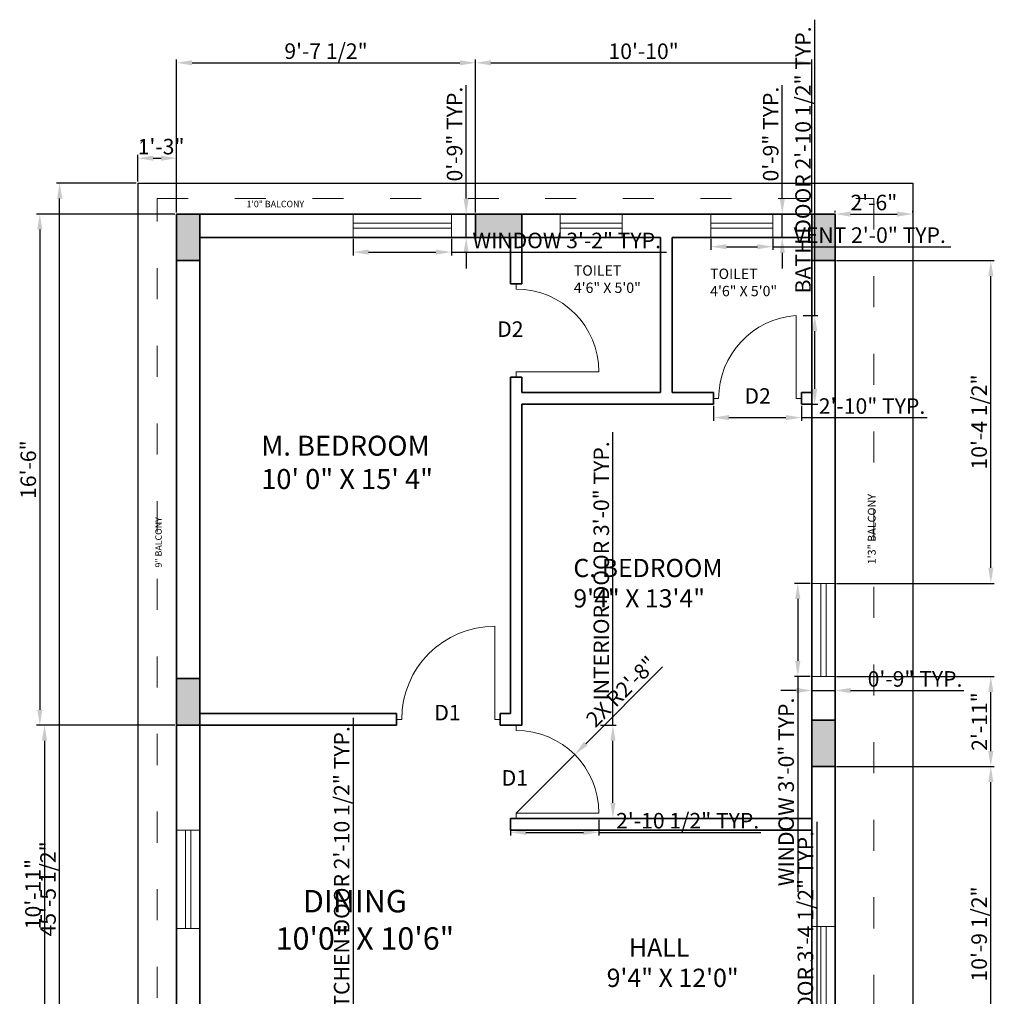
# Model space of a CAD drawing. Units: inches. Extents: x 40559 to 41508, y 131086 to 132358.
# Tile 4 of 5: x 41128 to 41508, y 131353 to 131730. Entities that reach past the tile are written whole.
import ezdxf

# ---------------------------------------------------------------- set-up
doc = ezdxf.new("R2010")
doc.units = ezdxf.units.IN
doc.linetypes.add('ACAD_ISO03W100', pattern=[30, 12, -18])
for name, color, linetype, lineweight in [('A-ANNO-DIMS', 2, 'Continuous', 18), ('A-ANNO-TEXT', 7, 'Continuous', 18), ('A-AREA-IDEN', 7, 'Continuous', 18), ('A-FLOR-FIXT', 4, 'Continuous', 18), ('A-FLOR-OVHD', 240, 'ACAD_ISO03W100', 13), ('A-WALL', 7, 'Continuous', 35), ('C-PROP', 7, 'Continuous', 25), ('Doors', 50, 'Continuous', 18), ('Windows', 70, 'Continuous', 18)]:
    doc.layers.add(name, color=color, linetype=linetype, lineweight=lineweight)
doc.layers.add('A-COLS', color=177, linetype='Continuous', lineweight=35, true_color=0x293189)
doc.styles.get("Standard").update_dxf_attribs({"font": 'arial.ttf'})
doc.dimstyles.new('ISO-25', dxfattribs={"dimtxt": 6, "dimasz": 6, "dimexe": 1.25, "dimexo": 0.625, "dimtad": 1, "dimdec": 0, "dimlunit": 3, "dimtxsty": 'Standard', "dimcen": 2.5, "dimclrd": 1, "dimclre": 1, "dimclrt": 2, "dimadec": 0, "dimazin": 0, "dimtfac": 1, "dimtdec": 0, "dimtmove": 0, "dimatfit": 3, "dimfxl": 1, "dimarcsym": 0})

# ---------------------------------------------------------------- blocks, each defined once
blk = doc.blocks.new('*D1')
at = {"layer": 'A-ANNO-DIMS', "color": 0, "lineweight": -2, "transparency": 16777216}
for p, q in [((41173.52, 131667.98), (41173.52, 131678.2)), ((41179.52, 131676.95), (41182.52, 131676.95)), ((41188.52, 131667.98), (41188.52, 131678.2))]:
    blk.add_line(p, q, dxfattribs=at)
at = {"layer": 'A-ANNO-DIMS', "color": 0, "transparency": 16777216}
for points in [[(41179.52, 131677.95), (41179.52, 131675.95), (41173.52, 131676.95)], [(41182.52, 131677.95), (41182.52, 131675.95), (41188.52, 131676.95)]]:
    blk.add_solid(points, dxfattribs=at)
at = {"layer": 'Defpoints', "color": 0, "transparency": 16777216}
for p in [(41188.52, 131676.95), (41173.52, 131667.35), (41188.52, 131667.35)]:
    blk.add_point(p, dxfattribs=at)
at = {"layer": 'A-ANNO-DIMS', "color": 0, "transparency": 16777216, "insert": (41182.52, 131680.64), "char_height": 6, "attachment_point": 5}
blk.add_mtext('1\'-3"', dxfattribs=at)
blk = doc.blocks.new('*D2')
at = {"layer": 'A-ANNO-DIMS', "color": 0, "lineweight": -2, "transparency": 16777216}
for p, q in [((41187.89, 131655.35), (41134.4, 131655.35)), ((41135.65, 131649.35), (41135.65, 131463.85)), ((41187.89, 131457.85), (41134.4, 131457.85))]:
    blk.add_line(p, q, dxfattribs=at)
at = {"layer": 'A-ANNO-DIMS', "color": 0, "transparency": 16777216}
for points in [[(41134.65, 131649.35), (41136.65, 131649.35), (41135.65, 131655.35)], [(41134.65, 131463.85), (41136.65, 131463.85), (41135.65, 131457.85)]]:
    blk.add_solid(points, dxfattribs=at)
at = {"layer": 'Defpoints', "color": 0, "transparency": 16777216}
for p in [(41188.52, 131655.35), (41135.65, 131457.85), (41188.52, 131457.85)]:
    blk.add_point(p, dxfattribs=at)
at = {"layer": 'A-ANNO-DIMS', "color": 0, "transparency": 16777216, "insert": (41131.96, 131556.6), "char_height": 6, "attachment_point": 5, "rotation": 90}
blk.add_mtext('16\'-6"', dxfattribs=at)
blk = doc.blocks.new('*D3')
at = {"layer": 'A-ANNO-DIMS', "color": 0, "lineweight": -2, "transparency": 16777216}
for p, q in [((41187.89, 131457.85), (41136.22, 131457.85)), ((41137.47, 131451.85), (41137.47, 131333.35)), ((41196.89, 131327.35), (41136.22, 131327.35))]:
    blk.add_line(p, q, dxfattribs=at)
at = {"layer": 'A-ANNO-DIMS', "color": 0, "transparency": 16777216}
for points in [[(41136.47, 131451.85), (41138.47, 131451.85), (41137.47, 131457.85)], [(41136.47, 131333.35), (41138.47, 131333.35), (41137.47, 131327.35)]]:
    blk.add_solid(points, dxfattribs=at)
at = {"layer": 'Defpoints', "color": 0, "transparency": 16777216}
for p in [(41188.52, 131457.85), (41137.47, 131327.35), (41197.52, 131327.35)]:
    blk.add_point(p, dxfattribs=at)
at = {"layer": 'A-ANNO-DIMS', "color": 0, "transparency": 16777216, "insert": (41133.78, 131392.6), "char_height": 6, "attachment_point": 5, "rotation": 90}
blk.add_mtext('10\'-11"', dxfattribs=at)
blk = doc.blocks.new('*D5')
at = {"layer": 'A-ANNO-DIMS', "color": 0, "lineweight": -2, "transparency": 16777216}
for p, q in [((41443.02, 131655.98), (41443.02, 131656.6)), ((41473.02, 131655.98), (41473.02, 131656.6)), ((41449.02, 131655.35), (41467.02, 131655.35))]:
    blk.add_line(p, q, dxfattribs=at)
at = {"layer": 'A-ANNO-DIMS', "color": 0, "transparency": 16777216}
for points in [[(41449.02, 131656.35), (41449.02, 131654.35), (41443.02, 131655.35)], [(41467.02, 131656.35), (41467.02, 131654.35), (41473.02, 131655.35)]]:
    blk.add_solid(points, dxfattribs=at)
at = {"layer": 'Defpoints', "color": 0, "transparency": 16777216}
for p in [(41443.02, 131655.35), (41473.02, 131655.35), (41473.02, 131655.35)]:
    blk.add_point(p, dxfattribs=at)
at = {"layer": 'A-ANNO-DIMS', "color": 0, "transparency": 16777216, "insert": (41458.02, 131659.04), "char_height": 6, "attachment_point": 5}
blk.add_mtext('2\'-6"', dxfattribs=at)
blk = doc.blocks.new('WIN-36IN')
for p, q in [((0, 5.5), (36, 5.5)), ((0, 3.5), (36, 3.5))]:
    blk.add_line(p, q)
blk.add_lwpolyline([(0, 9), (36, 9), (36, 0), (0, 0)], close=True)
blk = doc.blocks.new('WIN-38IN')
for p, q in [((0, 5.5), (38, 5.5)), ((0, 3.5), (38, 3.5))]:
    blk.add_line(p, q)
blk.add_lwpolyline([(0, 9), (38, 9), (38, 0), (0, 0)], close=True)
blk = doc.blocks.new('VENT-24IN')
for p, q in [((0, 5.5), (24, 5.5)), ((0, 3.5), (24, 3.5))]:
    blk.add_line(p, q)
blk.add_lwpolyline([(0, 9), (24, 9), (24, 0), (0, 0)], close=True)
blk = doc.blocks.new('DOOR-INT-36IN')
for p, q in [((2.25, 34), (2.25, 36)), ((4.5, 0), (0, 0)), ((2.25, 0), (2.25, 2)), ((2.25, 2), (34.25, 2))]:
    blk.add_line(p, q)
blk.add_arc((2.25, 2), 32, 0, 90)
blk = doc.blocks.new('DOOR-BATH-34IN')
for p, q in [((32, 2.25), (32, 34.25)), ((34, 4.5), (34, 0)), ((0, 2.25), (2, 2.25)), ((34, 2.25), (32, 2.25))]:
    blk.add_line(p, q)
blk.add_arc((34.07, 2.25), 32.07, 93.6952, 180)
blk = doc.blocks.new('DOOR-INT-40IN')
for p, q in [((38, 2.25), (38, 38.25)), ((40, 4.5), (40, 0)), ((2, 2.25), (0, 2.25)), ((40, 2.25), (38, 2.25))]:
    blk.add_line(p, q)
blk.add_arc((38, 2.25), 36, 90, 180)
blk = doc.blocks.new('COL-9X18IN')
h = blk.add_hatch(color=256)
h.dxf.hatch_style = 1
h.paths.add_polyline_path([(9, 18), (0, 18), (0, 0), (9, 0)])
blk.add_lwpolyline([(0, 18), (9, 18), (9, 0), (0, 0)], close=True)
blk = doc.blocks.new('*D34')
at = {"layer": 'A-ANNO-DIMS', "color": 1, "lineweight": -2, "transparency": 16777216}
for p, q in [((41433.39, 131512.67), (41427.37, 131512.67)), ((41428.62, 131506.67), (41428.62, 131482.67)), ((41433.39, 131476.67), (41427.37, 131476.67)), ((41428.62, 131476.67), (41428.62, 131393.5))]:
    blk.add_line(p, q, dxfattribs=at)
at = {"layer": 'A-ANNO-DIMS', "color": 1, "transparency": 16777216}
for points in [[(41427.62, 131506.67), (41429.62, 131506.67), (41428.62, 131512.67)], [(41427.62, 131482.67), (41429.62, 131482.67), (41428.62, 131476.67)]]:
    blk.add_solid(points, dxfattribs=at)
at = {"layer": 'Defpoints', "color": 0, "transparency": 16777216}
for p in [(41434.02, 131512.67), (41428.62, 131476.67), (41434.02, 131476.67)]:
    blk.add_point(p, dxfattribs=at)
at = {"layer": 'A-ANNO-DIMS', "color": 2, "transparency": 16777216, "insert": (41424.89, 131432.08), "char_height": 6, "attachment_point": 5, "rotation": 90}
blk.add_mtext('WINDOW 3\'-0" TYP.', dxfattribs=at)
blk = doc.blocks.new('*D35')
at = {"layer": 'A-ANNO-DIMS', "color": 1, "lineweight": -2, "transparency": 16777216}
for p, q in [((41434.02, 131476.05), (41434.02, 131470.02)), ((41443.02, 131476.05), (41443.02, 131470.02)), ((41428.02, 131471.27), (41422.02, 131471.27)), ((41434.02, 131471.27), (41443.02, 131471.27)), ((41449.02, 131471.27), (41492.84, 131471.27))]:
    blk.add_line(p, q, dxfattribs=at)
at = {"layer": 'A-ANNO-DIMS', "color": 1, "transparency": 16777216}
for points in [[(41428.02, 131472.27), (41428.02, 131470.27), (41434.02, 131471.27)], [(41449.02, 131472.27), (41449.02, 131470.27), (41443.02, 131471.27)]]:
    blk.add_solid(points, dxfattribs=at)
at = {"layer": 'Defpoints', "color": 0, "transparency": 16777216}
for p in [(41434.02, 131476.67), (41443.02, 131476.67), (41443.02, 131471.27)]:
    blk.add_point(p, dxfattribs=at)
at = {"layer": 'A-ANNO-DIMS', "color": 2, "transparency": 16777216, "insert": (41473.93, 131474.96), "char_height": 6, "attachment_point": 5}
blk.add_mtext('0\'-9" TYP.', dxfattribs=at)
blk = doc.blocks.new('*D36')
at = {"layer": 'A-ANNO-DIMS', "color": 1, "lineweight": -2, "transparency": 16777216}
for p, q in [((41256.73, 131645.73), (41256.73, 131639.4)), ((41294.73, 131645.73), (41294.73, 131639.4)), ((41262.73, 131640.65), (41288.73, 131640.65)), ((41294.73, 131640.65), (41377.9, 131640.65))]:
    blk.add_line(p, q, dxfattribs=at)
at = {"layer": 'A-ANNO-DIMS', "color": 1, "transparency": 16777216}
for points in [[(41262.73, 131641.65), (41262.73, 131639.65), (41256.73, 131640.65)], [(41288.73, 131641.65), (41288.73, 131639.65), (41294.73, 131640.65)]]:
    blk.add_solid(points, dxfattribs=at)
at = {"layer": 'Defpoints', "color": 0, "transparency": 16777216}
for p in [(41256.73, 131646.35), (41294.73, 131646.35), (41294.73, 131640.65)]:
    blk.add_point(p, dxfattribs=at)
at = {"layer": 'A-ANNO-DIMS', "color": 2, "transparency": 16777216, "insert": (41339.31, 131644.38), "char_height": 6, "attachment_point": 5}
blk.add_mtext('WINDOW 3\'-2" TYP.', dxfattribs=at)
blk = doc.blocks.new('*D37')
at = {"layer": 'A-ANNO-DIMS', "color": 1, "lineweight": -2, "transparency": 16777216}
for p, q in [((41300.43, 131661.35), (41300.43, 131705.17)), ((41295.35, 131655.35), (41301.68, 131655.35)), ((41300.43, 131646.35), (41300.43, 131655.35)), ((41295.35, 131646.35), (41301.68, 131646.35)), ((41300.43, 131640.35), (41300.43, 131634.35))]:
    blk.add_line(p, q, dxfattribs=at)
at = {"layer": 'A-ANNO-DIMS', "color": 1, "transparency": 16777216}
for points in [[(41299.43, 131661.35), (41301.43, 131661.35), (41300.43, 131655.35)], [(41299.43, 131640.35), (41301.43, 131640.35), (41300.43, 131646.35)]]:
    blk.add_solid(points, dxfattribs=at)
at = {"layer": 'Defpoints', "color": 0, "transparency": 16777216}
for p in [(41294.73, 131655.35), (41300.43, 131655.35), (41294.73, 131646.35)]:
    blk.add_point(p, dxfattribs=at)
at = {"layer": 'A-ANNO-DIMS', "color": 2, "transparency": 16777216, "insert": (41296.74, 131686.26), "char_height": 6, "attachment_point": 5, "rotation": 90}
blk.add_mtext('0\'-9" TYP.', dxfattribs=at)
blk = doc.blocks.new('*D38')
at = {"layer": 'A-ANNO-DIMS', "color": 1, "lineweight": -2, "transparency": 16777216}
for p, q in [((41395.02, 131645.73), (41395.02, 131641.5)), ((41419.02, 131645.73), (41419.02, 131641.5)), ((41401.02, 131642.75), (41413.02, 131642.75)), ((41419.02, 131642.75), (41487.83, 131642.75))]:
    blk.add_line(p, q, dxfattribs=at)
at = {"layer": 'A-ANNO-DIMS', "color": 1, "transparency": 16777216}
for points in [[(41401.02, 131643.75), (41401.02, 131641.75), (41395.02, 131642.75)], [(41413.02, 131643.75), (41413.02, 131641.75), (41419.02, 131642.75)]]:
    blk.add_solid(points, dxfattribs=at)
at = {"layer": 'Defpoints', "color": 0, "transparency": 16777216}
for p in [(41395.02, 131646.35), (41419.02, 131646.35), (41419.02, 131642.75)]:
    blk.add_point(p, dxfattribs=at)
at = {"layer": 'A-ANNO-DIMS', "color": 2, "transparency": 16777216, "insert": (41456.43, 131646.44), "char_height": 6, "attachment_point": 5}
blk.add_mtext('VENT 2\'-0" TYP.', dxfattribs=at)
blk = doc.blocks.new('*D39')
at = {"layer": 'A-ANNO-DIMS', "color": 1, "lineweight": -2, "transparency": 16777216}
for p, q in [((41422.62, 131661.35), (41422.62, 131705.17)), ((41419.64, 131655.35), (41423.87, 131655.35)), ((41422.62, 131646.35), (41422.62, 131655.35)), ((41419.64, 131646.35), (41423.87, 131646.35)), ((41422.62, 131640.35), (41422.62, 131634.35))]:
    blk.add_line(p, q, dxfattribs=at)
at = {"layer": 'A-ANNO-DIMS', "color": 1, "transparency": 16777216}
for points in [[(41421.62, 131661.35), (41423.62, 131661.35), (41422.62, 131655.35)], [(41421.62, 131640.35), (41423.62, 131640.35), (41422.62, 131646.35)]]:
    blk.add_solid(points, dxfattribs=at)
at = {"layer": 'Defpoints', "color": 0, "transparency": 16777216}
for p in [(41419.02, 131655.35), (41422.62, 131655.35), (41419.02, 131646.35)]:
    blk.add_point(p, dxfattribs=at)
at = {"layer": 'A-ANNO-DIMS', "color": 2, "transparency": 16777216, "insert": (41418.93, 131686.26), "char_height": 6, "attachment_point": 5, "rotation": 90}
blk.add_mtext('0\'-9" TYP.', dxfattribs=at)
blk = doc.blocks.new('*D40')
at = {"layer": 'A-ANNO-DIMS', "color": 1, "lineweight": -2, "transparency": 16777216}
for p, q in [((41357.17, 131457.85), (41357.17, 131571.09)), ((41352.39, 131457.85), (41358.42, 131457.85)), ((41357.17, 131427.85), (41357.17, 131451.85)), ((41352.39, 131421.85), (41358.42, 131421.85))]:
    blk.add_line(p, q, dxfattribs=at)
at = {"layer": 'A-ANNO-DIMS', "color": 1, "transparency": 16777216}
for points in [[(41356.17, 131451.85), (41358.17, 131451.85), (41357.17, 131457.85)], [(41356.17, 131427.85), (41358.17, 131427.85), (41357.17, 131421.85)]]:
    blk.add_solid(points, dxfattribs=at)
at = {"layer": 'Defpoints', "color": 0, "transparency": 16777216}
for p in [(41351.77, 131457.85), (41357.17, 131457.85), (41351.77, 131421.85)]:
    blk.add_point(p, dxfattribs=at)
at = {"layer": 'A-ANNO-DIMS', "color": 2, "transparency": 16777216, "insert": (41353.44, 131517.47), "char_height": 6, "attachment_point": 5, "rotation": 90}
blk.add_mtext('INTERIOR DOOR 3\'-0" TYP.', dxfattribs=at)
blk = doc.blocks.new('*D41')
at = {"layer": 'A-ANNO-DIMS', "color": 1, "lineweight": -2, "transparency": 16777216}
for p, q in [((41317.52, 131421.23), (41317.52, 131415.2)), ((41351.77, 131421.23), (41351.77, 131415.2)), ((41323.52, 131416.45), (41345.77, 131416.45)), ((41351.77, 131416.45), (41414.33, 131416.45))]:
    blk.add_line(p, q, dxfattribs=at)
at = {"layer": 'A-ANNO-DIMS', "color": 1, "transparency": 16777216}
for points in [[(41323.52, 131417.45), (41323.52, 131415.45), (41317.52, 131416.45)], [(41345.77, 131417.45), (41345.77, 131415.45), (41351.77, 131416.45)]]:
    blk.add_solid(points, dxfattribs=at)
at = {"layer": 'Defpoints', "color": 0, "transparency": 16777216}
for p in [(41317.52, 131421.85), (41351.77, 131421.85), (41351.77, 131416.45)]:
    blk.add_point(p, dxfattribs=at)
at = {"layer": 'A-ANNO-DIMS', "color": 2, "transparency": 16777216, "insert": (41386.05, 131420.18), "char_height": 6, "attachment_point": 5}
blk.add_mtext('2\'-10 1/2" TYP.', dxfattribs=at)
blk = doc.blocks.new('*D42')
at = {"layer": 'A-ANNO-DIMS', "color": 1, "lineweight": -2, "transparency": 16777216}
for p, q in [((41256.84, 131331.85), (41256.84, 131460.64)), ((41261.35, 131331.85), (41255.59, 131331.85)), ((41256.84, 131303.6), (41256.84, 131325.85)), ((41261.35, 131297.6), (41255.59, 131297.6))]:
    blk.add_line(p, q, dxfattribs=at)
at = {"layer": 'A-ANNO-DIMS', "color": 1, "transparency": 16777216}
for points in [[(41255.84, 131325.85), (41257.84, 131325.85), (41256.84, 131331.85)], [(41255.84, 131303.6), (41257.84, 131303.6), (41256.84, 131297.6)]]:
    blk.add_solid(points, dxfattribs=at)
at = {"layer": 'Defpoints', "color": 0, "transparency": 16777216}
for p in [(41256.84, 131331.85), (41261.98, 131331.85), (41261.98, 131297.6)]:
    blk.add_point(p, dxfattribs=at)
at = {"layer": 'A-ANNO-DIMS', "color": 2, "transparency": 16777216, "insert": (41253.11, 131399.25), "char_height": 6, "attachment_point": 5, "rotation": 90}
blk.add_mtext('KITCHEN DOOR 2\'-10 1/2" TYP.', dxfattribs=at)
blk = doc.blocks.new('*D44')
at = {"layer": 'A-ANNO-DIMS', "color": 1, "lineweight": -2, "transparency": 16777216}
for p, q in [((41436.09, 131304.85), (41436.09, 131420.55)), ((41430.64, 131304.85), (41437.34, 131304.85)), ((41436.09, 131270.35), (41436.09, 131298.85)), ((41430.64, 131264.35), (41437.34, 131264.35))]:
    blk.add_line(p, q, dxfattribs=at)
at = {"layer": 'A-ANNO-DIMS', "color": 1, "transparency": 16777216}
for points in [[(41435.09, 131298.85), (41437.09, 131298.85), (41436.09, 131304.85)], [(41435.09, 131270.35), (41437.09, 131270.35), (41436.09, 131264.35)]]:
    blk.add_solid(points, dxfattribs=at)
at = {"layer": 'Defpoints', "color": 0, "transparency": 16777216}
for p in [(41430.02, 131304.85), (41436.09, 131304.85), (41430.02, 131264.35)]:
    blk.add_point(p, dxfattribs=at)
at = {"layer": 'A-ANNO-DIMS', "color": 2, "transparency": 16777216, "insert": (41432.36, 131365.7), "char_height": 6, "attachment_point": 5, "rotation": 90}
blk.add_mtext('ENTRY DOOR 3\'-4 1/2" TYP.', dxfattribs=at)
blk = doc.blocks.new('*D46')
at = {"layer": 'A-ANNO-DIMS', "color": 1, "lineweight": -2, "transparency": 16777216}
for p, q in [((41435.15, 131616.1), (41435.15, 131730.46)), ((41430.64, 131616.1), (41436.4, 131616.1)), ((41435.15, 131587.85), (41435.15, 131610.1)), ((41430.64, 131581.85), (41436.4, 131581.85))]:
    blk.add_line(p, q, dxfattribs=at)
at = {"layer": 'A-ANNO-DIMS', "color": 1, "transparency": 16777216}
for points in [[(41434.15, 131610.1), (41436.15, 131610.1), (41435.15, 131616.1)], [(41434.15, 131587.85), (41436.15, 131587.85), (41435.15, 131581.85)]]:
    blk.add_solid(points, dxfattribs=at)
at = {"layer": 'Defpoints', "color": 0, "transparency": 16777216}
for p in [(41430.02, 131616.1), (41435.15, 131616.1), (41430.02, 131581.85)]:
    blk.add_point(p, dxfattribs=at)
at = {"layer": 'A-ANNO-DIMS', "color": 2, "transparency": 16777216, "insert": (41431.42, 131676.28), "char_height": 6, "attachment_point": 5, "rotation": 90}
blk.add_mtext('BATH DOOR 2\'-10 1/2" TYP.', dxfattribs=at)
blk = doc.blocks.new('*D47')
at = {"layer": 'A-ANNO-DIMS', "color": 1, "lineweight": -2, "transparency": 16777216}
for p, q in [((41396.02, 131581.23), (41396.02, 131575.46)), ((41430.02, 131581.23), (41430.02, 131575.46)), ((41402.02, 131576.71), (41424.02, 131576.71)), ((41430.02, 131576.71), (41478.6, 131576.71))]:
    blk.add_line(p, q, dxfattribs=at)
at = {"layer": 'A-ANNO-DIMS', "color": 1, "transparency": 16777216}
for points in [[(41402.02, 131577.71), (41402.02, 131575.71), (41396.02, 131576.71)], [(41424.02, 131577.71), (41424.02, 131575.71), (41430.02, 131576.71)]]:
    blk.add_solid(points, dxfattribs=at)
at = {"layer": 'Defpoints', "color": 0, "transparency": 16777216}
for p in [(41396.02, 131581.85), (41430.02, 131581.85), (41430.02, 131576.71)]:
    blk.add_point(p, dxfattribs=at)
at = {"layer": 'A-ANNO-DIMS', "color": 2, "transparency": 16777216, "insert": (41457.31, 131580.4), "char_height": 6, "attachment_point": 5}
blk.add_mtext('2\'-10" TYP.', dxfattribs=at)
blk = doc.blocks.new('*D72')
at = {"layer": 'A-ANNO-DIMS', "color": 1, "lineweight": -2, "transparency": 16777216}
for p, q in [((41172.89, 131667.35), (41142.07, 131667.35)), ((41143.32, 131127.85), (41143.32, 131661.35)), ((41172.89, 131121.85), (41142.07, 131121.85))]:
    blk.add_line(p, q, dxfattribs=at)
at = {"layer": 'A-ANNO-DIMS', "color": 1, "transparency": 16777216}
for points in [[(41142.32, 131661.35), (41144.32, 131661.35), (41143.32, 131667.35)], [(41142.32, 131127.85), (41144.32, 131127.85), (41143.32, 131121.85)]]:
    blk.add_solid(points, dxfattribs=at)
at = {"layer": 'Defpoints', "color": 0, "transparency": 16777216}
for p in [(41143.32, 131667.35), (41173.52, 131667.35), (41173.52, 131121.85)]:
    blk.add_point(p, dxfattribs=at)
at = {"layer": 'A-ANNO-DIMS', "color": 2, "transparency": 16777216, "insert": (41139.59, 131394.6), "char_height": 6, "attachment_point": 5, "rotation": 90}
blk.add_mtext('45\'-5 1/2"', dxfattribs=at)
blk = doc.blocks.new('*D73')
at = {"layer": 'A-ANNO-DIMS', "color": 1, "lineweight": -2, "transparency": 16777216}
for p, q in [((41188.52, 131655.98), (41188.52, 131715.05)), ((41194.52, 131713.8), (41298.02, 131713.8)), ((41304.02, 131655.98), (41304.02, 131715.05))]:
    blk.add_line(p, q, dxfattribs=at)
at = {"layer": 'A-ANNO-DIMS', "color": 1, "transparency": 16777216}
for points in [[(41194.52, 131714.8), (41194.52, 131712.8), (41188.52, 131713.8)], [(41298.02, 131714.8), (41298.02, 131712.8), (41304.02, 131713.8)]]:
    blk.add_solid(points, dxfattribs=at)
at = {"layer": 'Defpoints', "color": 0, "transparency": 16777216}
for p in [(41304.02, 131713.8), (41188.52, 131655.35), (41304.02, 131655.35)]:
    blk.add_point(p, dxfattribs=at)
at = {"layer": 'A-ANNO-DIMS', "color": 2, "transparency": 16777216, "insert": (41246.27, 131717.53), "char_height": 6, "attachment_point": 5}
blk.add_mtext('9\'-7 1/2"', dxfattribs=at)
blk = doc.blocks.new('*D74')
at = {"layer": 'A-ANNO-DIMS', "color": 1, "lineweight": -2, "transparency": 16777216}
for p, q in [((41304.02, 131655.98), (41304.02, 131715.05)), ((41310.02, 131713.8), (41428.02, 131713.8)), ((41434.02, 131655.98), (41434.02, 131715.05))]:
    blk.add_line(p, q, dxfattribs=at)
at = {"layer": 'A-ANNO-DIMS', "color": 1, "transparency": 16777216}
for points in [[(41310.02, 131714.8), (41310.02, 131712.8), (41304.02, 131713.8)], [(41428.02, 131714.8), (41428.02, 131712.8), (41434.02, 131713.8)]]:
    blk.add_solid(points, dxfattribs=at)
at = {"layer": 'Defpoints', "color": 0, "transparency": 16777216}
for p in [(41434.02, 131713.8), (41304.02, 131655.35), (41434.02, 131655.35)]:
    blk.add_point(p, dxfattribs=at)
at = {"layer": 'A-ANNO-DIMS', "color": 2, "transparency": 16777216, "insert": (41369.02, 131717.49), "char_height": 6, "attachment_point": 5}
blk.add_mtext('10\'-10"', dxfattribs=at)
blk = doc.blocks.new('*D77')
at = {"layer": 'A-ANNO-DIMS', "color": 1, "lineweight": -2, "transparency": 16777216}
for p, q in [((41443.64, 131441.85), (41504.47, 131441.85)), ((41503.22, 131318.51), (41503.22, 131435.85)), ((41443.64, 131312.51), (41504.47, 131312.51))]:
    blk.add_line(p, q, dxfattribs=at)
at = {"layer": 'A-ANNO-DIMS', "color": 1, "transparency": 16777216}
for points in [[(41502.22, 131435.85), (41504.22, 131435.85), (41503.22, 131441.85)], [(41502.22, 131318.51), (41504.22, 131318.51), (41503.22, 131312.51)]]:
    blk.add_solid(points, dxfattribs=at)
at = {"layer": 'Defpoints', "color": 0, "transparency": 16777216}
for p in [(41443.02, 131441.85), (41503.22, 131441.85), (41443.02, 131312.51)]:
    blk.add_point(p, dxfattribs=at)
at = {"layer": 'A-ANNO-DIMS', "color": 2, "transparency": 16777216, "insert": (41499.49, 131377.18), "char_height": 6, "attachment_point": 5, "rotation": 90}
blk.add_mtext('10\'-9 1/2"', dxfattribs=at)
blk = doc.blocks.new('*D78')
at = {"layer": 'A-ANNO-DIMS', "color": 1, "lineweight": -2, "transparency": 16777216}
for p, q in [((41443.64, 131476.67), (41504.47, 131476.67)), ((41503.22, 131447.85), (41503.22, 131470.67)), ((41443.64, 131441.85), (41504.47, 131441.85))]:
    blk.add_line(p, q, dxfattribs=at)
at = {"layer": 'A-ANNO-DIMS', "color": 1, "transparency": 16777216}
for points in [[(41502.22, 131470.67), (41504.22, 131470.67), (41503.22, 131476.67)], [(41502.22, 131447.85), (41504.22, 131447.85), (41503.22, 131441.85)]]:
    blk.add_solid(points, dxfattribs=at)
at = {"layer": 'Defpoints', "color": 0, "transparency": 16777216}
for p in [(41443.02, 131476.67), (41503.22, 131476.67), (41443.02, 131441.85)]:
    blk.add_point(p, dxfattribs=at)
at = {"layer": 'A-ANNO-DIMS', "color": 2, "transparency": 16777216, "insert": (41499.58, 131459.26), "char_height": 6, "attachment_point": 5, "rotation": 90}
blk.add_mtext('2\'-11"', dxfattribs=at)
blk = doc.blocks.new('*D79')
at = {"layer": 'A-ANNO-DIMS', "color": 1, "lineweight": -2, "transparency": 16777216}
for p, q in [((41443.64, 131637.35), (41504.47, 131637.35)), ((41503.22, 131518.67), (41503.22, 131631.35)), ((41443.64, 131512.67), (41504.47, 131512.67))]:
    blk.add_line(p, q, dxfattribs=at)
at = {"layer": 'A-ANNO-DIMS', "color": 1, "transparency": 16777216}
for points in [[(41502.22, 131631.35), (41504.22, 131631.35), (41503.22, 131637.35)], [(41502.22, 131518.67), (41504.22, 131518.67), (41503.22, 131512.67)]]:
    blk.add_solid(points, dxfattribs=at)
at = {"layer": 'Defpoints', "color": 0, "transparency": 16777216}
for p in [(41443.02, 131637.35), (41503.22, 131637.35), (41443.02, 131512.67)]:
    blk.add_point(p, dxfattribs=at)
at = {"layer": 'A-ANNO-DIMS', "color": 2, "transparency": 16777216, "insert": (41499.49, 131575.01), "char_height": 6, "attachment_point": 5, "rotation": 90}
blk.add_mtext('10\'-4 1/2"', dxfattribs=at)
blk = doc.blocks.new('*D105')
at = {"layer": 'A-ANNO-DIMS', "color": 1, "lineweight": -2, "transparency": 16777216}
for p, q in [((41376.29, 131480.37), (41346.64, 131450.72)), ((41319.77, 131423.85), (41342.39, 131446.48))]:
    blk.add_line(p, q, dxfattribs=at)
at = {"layer": 'A-ANNO-DIMS', "color": 1, "transparency": 16777216}
blk.add_solid([(41345.93, 131451.43), (41347.34, 131450.01), (41342.39, 131446.48)], dxfattribs=at)
at = {"layer": 'Defpoints', "color": 0, "transparency": 16777216}
for p in [(41342.39, 131446.48), (41319.77, 131423.85)]:
    blk.add_point(p, dxfattribs=at)
at = {"layer": 'A-ANNO-DIMS', "color": 2, "transparency": 16777216, "insert": (41360.98, 131470.28), "char_height": 6, "attachment_point": 5, "rotation": 45.0006}
blk.add_mtext('2X R2\'-8"', dxfattribs=at)

msp = doc.modelspace()

# ---------------------------------------------------------------- linework, layer by layer
at = {"layer": 'A-FLOR-FIXT', "extrusion": (0, 0, -1)}
msp.add_ellipse((41174.58, 131683.6), major_axis=(0, 0.841), ratio=0.888017, start_param=1.570796, end_param=3.141593, dxfattribs=at)
msp.add_ellipse((41174.58, 131683.6), major_axis=(0, 0.841), ratio=0.888017, start_param=1.570796, end_param=3.141593, dxfattribs=at)
at = {"layer": 'A-FLOR-OVHD'}
for p, q in [((41181.02, 131202.46), (41181.02, 131661.35)), ((41181.02, 131661.35), (41458.02, 131661.35)), ((41458.02, 131661.35), (41458.02, 131121.85))]:
    msp.add_line(p, q, dxfattribs=at)
at = {"layer": 'A-WALL'}
for p, q in [((41188.52, 131655.35), (41188.52, 131198.35)), ((41188.52, 131655.35), (41443.02, 131655.35)), ((41443.02, 131655.35), (41443.02, 131264.35)), ((41197.52, 131646.35), (41317.52, 131646.35)), ((41197.52, 131646.35), (41197.52, 131207.35)), ((41197.52, 131646.35), (41317.52, 131646.35)), ((41317.52, 131646.35), (41317.52, 131628.35)), ((41322.02, 131646.35), (41322.02, 131628.35)), ((41322.02, 131646.35), (41375.52, 131646.35)), ((41322.02, 131646.35), (41375.52, 131646.35)), ((41375.52, 131646.35), (41375.52, 131586.35)), ((41380.02, 131646.35), (41380.02, 131586.35)), ((41380.02, 131646.35), (41434.02, 131646.35)), ((41380.02, 131646.35), (41434.02, 131646.35)), ((41434.02, 131646.35), (41434.02, 131273.35)), ((41434.02, 131646.35), (41434.02, 131586.35)), ((41317.52, 131628.35), (41322.02, 131628.35)), ((41322.02, 131592.35), (41317.52, 131592.35)), ((41317.52, 131592.35), (41317.52, 131462.35)), ((41322.02, 131592.35), (41322.02, 131586.35)), ((41322.02, 131586.35), (41375.52, 131586.35)), ((41380.02, 131586.35), (41396.02, 131586.35)), ((41396.02, 131586.35), (41396.02, 131581.85)), ((41430.02, 131586.35), (41430.02, 131581.85)), ((41430.02, 131586.35), (41434.02, 131586.35)), ((41322.02, 131581.85), (41396.02, 131581.85)), ((41322.02, 131581.85), (41322.02, 131457.85)), ((41430.02, 131581.85), (41434.02, 131581.85)), ((41197.52, 131462.35), (41273.52, 131462.35)), ((41273.52, 131462.35), (41273.52, 131457.85)), ((41313.52, 131462.35), (41313.52, 131457.85)), ((41313.52, 131462.35), (41317.52, 131462.35)), ((41197.52, 131457.85), (41273.52, 131457.85)), ((41313.52, 131457.85), (41317.52, 131457.85)), ((41317.52, 131457.85), (41322.02, 131457.85)), ((41317.52, 131421.85), (41434.02, 131421.85)), ((41317.52, 131421.85), (41317.52, 131417.35)), ((41317.52, 131417.35), (41434.02, 131417.35))]:
    msp.add_line(p, q, dxfattribs=at)
at = {"layer": 'C-PROP'}
for p, q in [((41173.52, 131667.35), (41173.52, 131121.85)), ((41173.52, 131667.35), (41473.02, 131667.35)), ((41473.02, 131667.35), (41473.02, 131121.85))]:
    msp.add_line(p, q, dxfattribs=at)

# ---------------------------------------------------------------- block references
at = {"layer": 'A-COLS'}
for p in [(41188.52, 131637.35), (41188.52, 131457.85)]:
    msp.add_blockref('COL-9X18IN', p, dxfattribs=at)
for p, rotation in [((41304.02, 131655.35), 270.0000000000275), ((41443.02, 131655.35), 180), ((41443.02, 131459.85), 180)]:
    msp.add_blockref('COL-9X18IN', p, dxfattribs=dict(at, rotation=rotation))
at = {"layer": 'Doors'}
for name, p in [('DOOR-INT-36IN', (41317.52, 131592.35)), ('DOOR-BATH-34IN', (41396.02, 131581.85)), ('DOOR-INT-40IN', (41273.52, 131457.85)), ('DOOR-INT-36IN', (41317.52, 131421.85))]:
    msp.add_blockref(name, p, dxfattribs=at)
at = {"layer": 'Windows'}
for name, p in [('WIN-38IN', (41256.73, 131646.35)), ('VENT-24IN', (41336.77, 131646.35)), ('VENT-24IN', (41395.02, 131646.35))]:
    msp.add_blockref(name, p, dxfattribs=at)
for name, p, rotation in [('WIN-36IN', (41434.02, 131512.67), 269.9999999999951), ('WIN-38IN', (41188.52, 131417.3), 269.9999999999867), ('WIN-38IN', (41434.02, 131380.06), 269.9999999999867)]:
    msp.add_blockref(name, p, dxfattribs=dict(at, rotation=rotation))

# ---------------------------------------------------------------- texts
at = {"layer": 'A-ANNO-TEXT', "attachment_point": 1}
for s, width, insert, char_height in [('{\\fArial|b1|i0|c0|p34;1\'0" BALCONY}', 44.482, (41215.54, 131660.49), 2.5), ('{D2}', 6, (41312.43, 131613.89), 6), ('{D2}', 6, (41408, 131588.07), 6), ('{D1}', 6, (41288.13, 131465.71), 6), ('{D1}', 6, (41314.17, 131440.49), 6)]:
    msp.add_mtext_dynamic_manual_height_columns(s, width=width, gutter_width=12.5, heights=[0], dxfattribs=dict(at, insert=insert, char_height=char_height))
at = {"layer": 'A-ANNO-TEXT', "attachment_point": 1, "rotation": 90}
for s, width, gutter_width, insert, char_height in [('{\\fArial|b1|i0|c0|p34;1\'3" BALCONY}', 32.0122, 15.27, (41455.68, 131520), 3.0532), ('{\\fArial|b1|i0|c0|p34;9" BALCONY}', 44.482, 12.5, (41180.28, 131518.8), 2.5)]:
    msp.add_mtext_dynamic_manual_height_columns(s, width=width, gutter_width=gutter_width, heights=[0], dxfattribs=dict(at, insert=insert, char_height=char_height))
at = {"layer": 'A-AREA-IDEN', "attachment_point": 1}
for s, width, gutter_width, insert, char_height in [('{\\fArial|b1|i0|c0|p34;TOILET\\P4\'6" X 5\'0"}', 37.2303, 12.5, (41342.05, 131635.55), 4), ('{\\fArial|b1|i0|c0|p34;TOILET\\P4\'6" X 5\'0"}', 37.2303, 12.5, (41394.74, 131634.28), 4), ('{\\fArial|b1|i0|c0|p34;M. BEDROOM\\P10\' 0" X 15\' 4"}', 78.1402, 16.09, (41221.22, 131569.71), 7.7236), ('{\\fArial|b1|i0|c0|p34;C. BEDROOM\\P9\'4" X 13\'4"}', 75.8875, 14.66, (41341.87, 131522.12), 7.0382), ('{\\fArial|b1|i0|c0|p34;    DINING\\P10\'0" X 10\'6"}', 98.8896, 43.2, (41226.79, 131394.17), 8.639), ('{\\fArial|b1|i0|c0|p34;    HALL\\P9\'4" X 12\'0"}', 82.7784, 14.7, (41354.74, 131375.53), 7.0565)]:
    msp.add_mtext_dynamic_manual_height_columns(s, width=width, gutter_width=gutter_width, heights=[0], dxfattribs=dict(at, insert=insert, char_height=char_height))

# ---------------------------------------------------------------- dimensions: what is measured, and where the dimension line sits
at = {"layer": 'A-ANNO-DIMS'}
for base, p1, p2, angle, text, picture, middle in [((41435.15435623, 131616.10041044), (41430.01685623, 131581.85041044), (41430.01685623, 131616.10041044), 90, 'BATH DOOR <> TYP.', '*D46', (41431.42499061, 131676.27929857)), ((41300.43, 131655.35), (41294.73, 131646.35), (41294.73, 131655.35), 90, '<> TYP.', '*D37', (41296.74, 131686.26)), ((41422.62, 131655.35), (41419.02, 131646.35), (41419.02, 131655.35), 90, '<> TYP.', '*D39', (41418.93, 131686.26)), ((41357.17, 131457.85), (41351.77, 131421.85), (41351.77, 131457.85), 90, 'INTERIOR DOOR <> TYP.', '*D40', (41353.44, 131517.47)), ((41428.62, 131476.67), (41434.02, 131512.67), (41434.02, 131476.67), 270, 'WINDOW <> TYP.', '*D34', (41424.89, 131432.08)), ((41256.83955995, 131331.85041044), (41261.97705995, 131297.60041044), (41261.97705995, 131331.85041044), 90, 'KITCHEN DOOR <> TYP.', '*D42', (41253.11019433, 131399.24689748)), ((41436.09, 131304.85), (41430.02, 131264.35), (41430.02, 131304.85), 90, 'ENTRY DOOR <> TYP.', '*D44', (41432.36, 131365.7))]:
    dim = msp.add_linear_dim(base=base, p1=p1, p2=p2, angle=angle, text=text, dimstyle='ISO-25', override={"dimdec": 1, "dimlfac": 1, "dimrnd": 0, "dimzin": 1, "dimdsep": 46, "dimlunit": 4, "dimfrac": 2}, dxfattribs=at)
    dim.commit()
    dim.dimension.update_dxf_attribs({"geometry": picture, "text_midpoint": middle})
for base, p1, p2, override, picture, middle in [((41304.02, 131713.8), (41188.52, 131655.35), (41304.02, 131655.35), {"dimdec": 1, "dimlfac": 1, "dimrnd": 0, "dimzin": 1, "dimdsep": 46, "dimlunit": 4, "dimfrac": 2}, '*D73', (41246.27, 131717.53)), ((41434.02, 131713.8), (41304.02, 131655.35), (41434.02, 131655.35), {"dimdec": 1, "dimlfac": 1, "dimrnd": 0, "dimzin": 1, "dimdsep": 46, "dimlunit": 4, "dimfrac": 2}, '*D74', (41369.02, 131717.49)), ((41473.02, 131655.35), (41443.02, 131655.35), (41473.02, 131655.35), {"dimclrd": 0, "dimclre": 0, "dimclrt": 0}, '*D5', (41458.02, 131659.04))]:
    dim = msp.add_linear_dim(base=base, p1=p1, p2=p2, dimstyle='ISO-25', override=override, dxfattribs=at)
    dim.commit()
    dim.dimension.update_dxf_attribs({"geometry": picture, "text_midpoint": middle})
dim = msp.add_linear_dim(base=(41188.52, 131676.95), p1=(41173.52, 131667.35), p2=(41188.52, 131667.35), dimstyle='ISO-25', override={"dimclrd": 0, "dimclre": 0, "dimclrt": 0}, dxfattribs=at)
dim.commit()
dim.dimension.update_dxf_attribs({"geometry": '*D1', "text_midpoint": (41182.52, 131676.95), "dimtype": 160})
for base, p1, p2, override, picture, middle in [((41143.32, 131667.35), (41173.52, 131121.85), (41173.52, 131667.35), {"dimdec": 1, "dimlfac": 1, "dimrnd": 0, "dimzin": 1, "dimdsep": 46, "dimlunit": 4, "dimfrac": 2}, '*D72', (41139.59, 131394.6)), ((41135.6504808, 131457.85041044), (41188.51685623, 131655.35041044), (41188.51685623, 131457.85041044), {"dimclrd": 0, "dimclre": 0, "dimclrt": 0}, '*D2', (41131.96204287, 131556.60041044)), ((41503.22, 131637.35), (41443.02, 131512.67), (41443.02, 131637.35), {"dimdec": 1, "dimlfac": 1, "dimrnd": 0, "dimzin": 1, "dimdsep": 46, "dimlunit": 4, "dimfrac": 2}, '*D79', (41499.49, 131575.01)), ((41503.22, 131476.67), (41443.02, 131441.85), (41443.02, 131476.67), {"dimdec": 1, "dimlfac": 1, "dimrnd": 0, "dimzin": 1, "dimdsep": 46, "dimlunit": 4, "dimfrac": 2}, '*D78', (41499.58, 131459.26)), ((41137.46517777, 131327.35041044), (41188.51685623, 131457.85041044), (41197.51685623, 131327.35041044), {"dimclrd": 0, "dimclre": 0, "dimclrt": 0}, '*D3', (41133.77673984, 131392.60041044)), ((41503.22, 131441.85), (41443.02, 131312.51), (41443.02, 131441.85), {"dimdec": 1, "dimlfac": 1, "dimrnd": 0, "dimzin": 1, "dimdsep": 46, "dimlunit": 4, "dimfrac": 2}, '*D77', (41499.49, 131377.18))]:
    dim = msp.add_linear_dim(base=base, p1=p1, p2=p2, angle=90, dimstyle='ISO-25', override=override, dxfattribs=at)
    dim.commit()
    dim.dimension.update_dxf_attribs({"geometry": picture, "text_midpoint": middle})
for base, p1, p2, text, picture, middle in [((41419.02, 131642.75), (41395.02, 131646.35), (41419.02, 131646.35), 'VENT <> TYP.', '*D38', (41456.43, 131646.44)), ((41294.73, 131640.65), (41256.73, 131646.35), (41294.73, 131646.35), 'WINDOW <> TYP.', '*D36', (41339.31, 131644.38)), ((41430.02, 131576.71), (41396.02, 131581.85), (41430.02, 131581.85), '<> TYP.', '*D47', (41457.31, 131580.4)), ((41443.02, 131471.27), (41434.02, 131476.67), (41443.02, 131476.67), '<> TYP.', '*D35', (41473.93, 131474.96)), ((41351.76685623, 131416.45041044), (41317.51685623, 131421.85041044), (41351.76685623, 131421.85041044), '<> TYP.', '*D41', (41386.05079211, 131420.17772968))]:
    dim = msp.add_linear_dim(base=base, p1=p1, p2=p2, text=text, dimstyle='ISO-25', override={"dimdec": 1, "dimlfac": 1, "dimrnd": 0, "dimzin": 1, "dimdsep": 46, "dimlunit": 4, "dimfrac": 2}, dxfattribs=at)
    dim.commit()
    dim.dimension.update_dxf_attribs({"geometry": picture, "text_midpoint": middle})
dim = msp.add_radius_dim(center=(41319.77, 131423.85), mpoint=(41342.39, 131446.48), text='2X <>', dimstyle='ISO-25', override={"dimdec": 1, "dimlfac": 1, "dimrnd": 0, "dimzin": 1, "dimdsep": 46, "dimlunit": 4, "dimfrac": 2}, dxfattribs=at)
dim.commit()
dim.dimension.update_dxf_attribs({"geometry": '*D105', "text_midpoint": (41360.98, 131470.28)})

doc.saveas('drawing.dxf')
